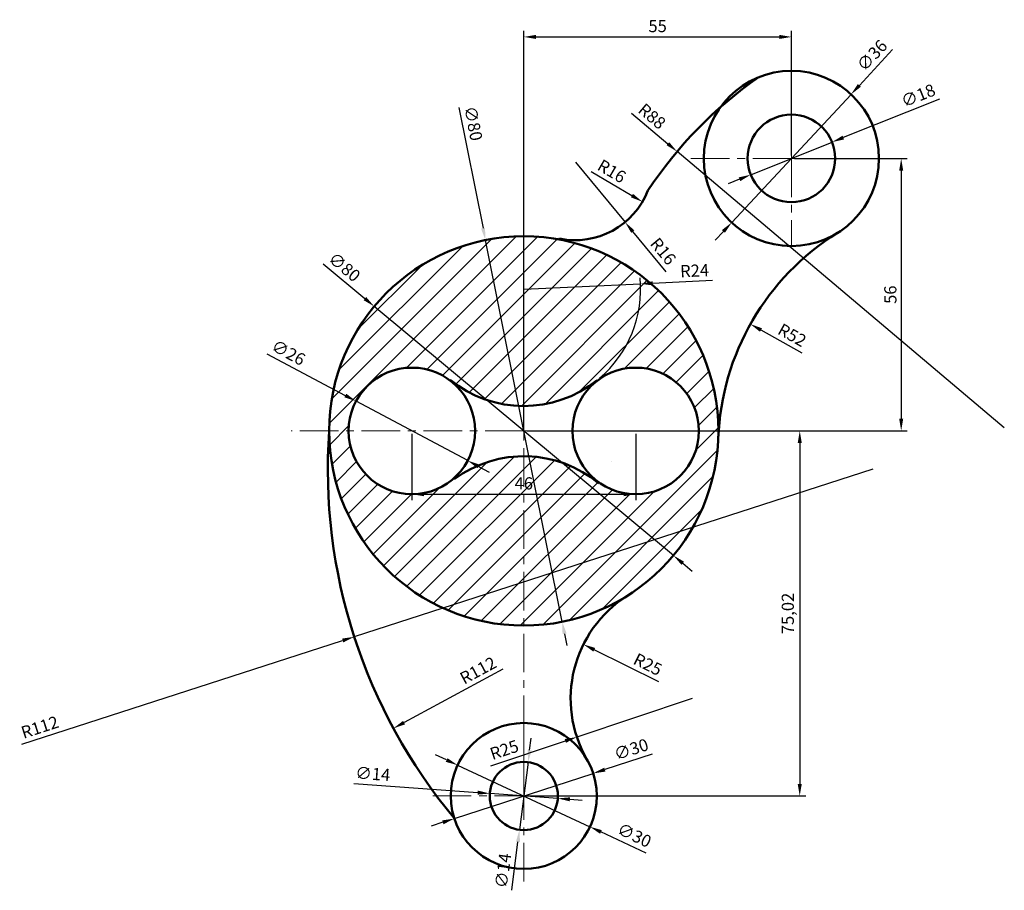
# Model space of a CAD drawing. Units: millimetres. Extents: x 2710 to 2913, y 1178 to 1357.
import ezdxf

# ---------------------------------------------------------------- set-up
doc = ezdxf.new("R2010")
doc.units = ezdxf.units.MM
doc.linetypes.add('CENTER', pattern=[50.8, 31.75, -6.35, 6.35, -6.35])
for name, color, linetype, lineweight in [('M-CNTR', 4, 'CENTER', 18), ('M-DIMS', 2, 'Continuous', 25), ('M-HATC', 8, 'Continuous', 18), ('M-OUTL', 7, 'Continuous', 50)]:
    doc.layers.add(name, color=color, linetype=linetype, lineweight=lineweight)
doc.styles.get("Standard").update_dxf_attribs({"font": 'arial.ttf'})
doc.dimstyles.new('ISO-25', dxfattribs={"dimtxt": 2.5, "dimasz": 2.5, "dimexe": 1.25, "dimexo": 0.625, "dimtad": 1, "dimtxsty": 'Standard', "dimcen": 2.5, "dimadec": 0, "dimazin": 0, "dimtfac": 1, "dimtmove": 0, "dimatfit": 3, "dimfxl": 1, "dimarcsym": 0})

# ---------------------------------------------------------------- blocks, each defined once
blk = doc.blocks.new('*D1')
at = {"layer": 'Defpoints', "color": 0, "transparency": 16777216}
for p in [(2813.89, 1272.64), (2813.89, 1197.62), (2870.6, 1197.62)]:
    blk.add_point(p, dxfattribs=at)
at = {"layer": 'M-DIMS', "color": 0, "lineweight": -2, "transparency": 16777216}
for p, q in [((2814.51, 1272.64), (2871.85, 1272.64)), ((2870.6, 1270.14), (2870.6, 1200.12)), ((2814.51, 1197.62), (2871.85, 1197.62))]:
    blk.add_line(p, q, dxfattribs=at)
at = {"layer": 'M-DIMS', "color": 0, "transparency": 16777216}
for points in [[(2870.18, 1270.14), (2871.02, 1270.14), (2870.6, 1272.64)], [(2870.18, 1200.12), (2871.02, 1200.12), (2870.6, 1197.62)]]:
    blk.add_solid(points, dxfattribs=at)
at = {"layer": 'M-DIMS', "color": 0, "transparency": 16777216, "insert": (2868.47, 1235.13), "char_height": 2.5, "attachment_point": 5, "rotation": 90}
blk.add_mtext('75,02', dxfattribs=at)
blk = doc.blocks.new('*D2')
at = {"layer": 'Defpoints', "color": 0, "transparency": 16777216}
for p in [(2868.89, 1353.61), (2868.89, 1328.64), (2813.89, 1272.64)]:
    blk.add_point(p, dxfattribs=at)
at = {"layer": 'M-DIMS', "color": 0, "lineweight": -2, "transparency": 16777216}
for p, q in [((2813.89, 1273.27), (2813.89, 1354.86)), ((2868.89, 1329.27), (2868.89, 1354.86)), ((2816.39, 1353.61), (2866.39, 1353.61))]:
    blk.add_line(p, q, dxfattribs=at)
at = {"layer": 'M-DIMS', "color": 0, "transparency": 16777216}
for points in [[(2816.39, 1354.03), (2816.39, 1353.19), (2813.89, 1353.61)], [(2866.39, 1354.03), (2866.39, 1353.19), (2868.89, 1353.61)]]:
    blk.add_solid(points, dxfattribs=at)
at = {"layer": 'M-DIMS', "color": 0, "transparency": 16777216, "insert": (2841.39, 1355.51), "char_height": 2.5, "attachment_point": 5}
blk.add_mtext('55', dxfattribs=at)
blk = doc.blocks.new('*D3')
at = {"layer": 'Defpoints', "color": 0, "transparency": 16777216}
for p in [(2868.89, 1328.64), (2813.89, 1272.64), (2891.45, 1272.64)]:
    blk.add_point(p, dxfattribs=at)
at = {"layer": 'M-DIMS', "color": 0, "lineweight": -2, "transparency": 16777216}
for p, q in [((2869.51, 1328.64), (2892.7, 1328.64)), ((2891.45, 1326.14), (2891.45, 1275.14)), ((2814.51, 1272.64), (2892.7, 1272.64))]:
    blk.add_line(p, q, dxfattribs=at)
at = {"layer": 'M-DIMS', "color": 0, "transparency": 16777216}
for points in [[(2891.04, 1326.14), (2891.87, 1326.14), (2891.45, 1328.64)], [(2891.04, 1275.14), (2891.87, 1275.14), (2891.45, 1272.64)]]:
    blk.add_solid(points, dxfattribs=at)
at = {"layer": 'M-DIMS', "color": 0, "transparency": 16777216, "insert": (2889.55, 1300.64), "char_height": 2.5, "attachment_point": 5, "rotation": 90}
blk.add_mtext('56', dxfattribs=at)
blk = doc.blocks.new('*D4')
at = {"layer": 'Defpoints', "color": 0, "transparency": 16777216}
for p in [(2813.89, 1301.75), (2837.86, 1302.86)]:
    blk.add_point(p, dxfattribs=at)
at = {"layer": 'M-DIMS', "color": 0, "lineweight": -2, "transparency": 16777216}
for p, q in [((2852.69, 1303.54), (2840.36, 1302.97)), ((2813.89, 1301.75), (2837.86, 1302.86))]:
    blk.add_line(p, q, dxfattribs=at)
blk.add_arc((2813.89, 1301.75), 24, 310.331, 5.6178, dxfattribs=at)
at = {"layer": 'M-DIMS', "color": 0, "transparency": 16777216}
blk.add_solid([(2840.34, 1303.39), (2840.38, 1302.56), (2837.86, 1302.86)], dxfattribs=at)
at = {"layer": 'M-DIMS', "color": 0, "transparency": 16777216, "insert": (2849, 1305.25), "char_height": 2.5, "attachment_point": 5, "rotation": 2.6336}
blk.add_mtext('R24', dxfattribs=at)
blk = doc.blocks.new('*D5')
at = {"layer": 'Defpoints', "color": 0, "transparency": 16777216}
for p in [(2826.14, 1228.78), (2848.52, 1217.64)]:
    blk.add_point(p, dxfattribs=at)
at = {"layer": 'M-DIMS', "color": 0, "lineweight": -2, "transparency": 16777216}
blk.add_line((2841.64, 1221.06), (2828.38, 1227.67), dxfattribs=at)
at = {"layer": 'M-DIMS', "color": 0, "transparency": 16777216}
blk.add_solid([(2828.57, 1228.04), (2828.19, 1227.29), (2826.14, 1228.78)], dxfattribs=at)
at = {"layer": 'M-DIMS', "color": 0, "transparency": 16777216, "insert": (2839.24, 1224.38), "char_height": 2.5, "attachment_point": 5, "rotation": 333.5253}
blk.add_mtext('R25', dxfattribs=at)
blk = doc.blocks.new('*D6')
at = {"layer": 'Defpoints', "color": 0, "transparency": 16777216}
for p in [(2885.61, 1264.77), (2787.08, 1211.52)]:
    blk.add_point(p, dxfattribs=at)
at = {"layer": 'M-DIMS', "color": 0, "lineweight": -2, "transparency": 16777216}
blk.add_line((2809.55, 1223.66), (2789.28, 1212.71), dxfattribs=at)
at = {"layer": 'M-DIMS', "color": 0, "transparency": 16777216}
blk.add_solid([(2789.08, 1213.07), (2789.47, 1212.34), (2787.08, 1211.52)], dxfattribs=at)
at = {"layer": 'M-DIMS', "color": 0, "transparency": 16777216, "insert": (2804.64, 1223.15), "char_height": 2.5, "attachment_point": 5, "rotation": 28.3886}
blk.add_mtext('R112', dxfattribs=at)
blk = doc.blocks.new('*D7')
at = {"layer": 'Defpoints', "color": 0, "transparency": 16777216}
for p in [(2824.48, 1327.84), (2838.27, 1319.73)]:
    blk.add_point(p, dxfattribs=at)
at = {"layer": 'M-DIMS', "color": 0, "lineweight": -2, "transparency": 16777216}
blk.add_line((2827.74, 1325.93), (2836.12, 1321), dxfattribs=at)
at = {"layer": 'M-DIMS', "color": 0, "transparency": 16777216}
blk.add_solid([(2836.33, 1321.36), (2835.91, 1320.64), (2838.27, 1319.73)], dxfattribs=at)
at = {"layer": 'M-DIMS', "color": 0, "transparency": 16777216, "insert": (2831.81, 1325.74), "char_height": 2.5, "attachment_point": 5, "rotation": 329.5523}
blk.add_mtext('R16', dxfattribs=at)
blk = doc.blocks.new('*D8')
at = {"layer": 'Defpoints', "color": 0, "transparency": 16777216}
for p in [(2845.4, 1330.05), (2912.65, 1273.29)]:
    blk.add_point(p, dxfattribs=at)
at = {"layer": 'M-DIMS', "color": 0, "lineweight": -2, "transparency": 16777216}
for p, q in [((2836.05, 1337.94), (2843.49, 1331.66)), ((2912.65, 1273.29), (2845.4, 1330.05))]:
    blk.add_line(p, q, dxfattribs=at)
at = {"layer": 'M-DIMS', "color": 0, "transparency": 16777216}
blk.add_solid([(2843.76, 1331.98), (2843.22, 1331.35), (2845.4, 1330.05)], dxfattribs=at)
at = {"layer": 'M-DIMS', "color": 0, "transparency": 16777216, "insert": (2840.04, 1337.06), "char_height": 2.5, "attachment_point": 5, "rotation": 319.8348}
blk.add_mtext('R88', dxfattribs=at)
blk = doc.blocks.new('*D9')
at = {"layer": 'Defpoints', "color": 0, "transparency": 16777216}
for p in [(2860.46, 1294.59), (2905.82, 1269.18)]:
    blk.add_point(p, dxfattribs=at)
at = {"layer": 'M-DIMS', "color": 0, "lineweight": -2, "transparency": 16777216}
blk.add_line((2871.1, 1288.63), (2862.64, 1293.37), dxfattribs=at)
at = {"layer": 'M-DIMS', "color": 0, "transparency": 16777216}
blk.add_solid([(2862.84, 1293.74), (2862.43, 1293.01), (2860.46, 1294.59)], dxfattribs=at)
at = {"layer": 'M-DIMS', "color": 0, "transparency": 16777216, "insert": (2868.89, 1292.05), "char_height": 2.5, "attachment_point": 5, "rotation": 330.7397}
blk.add_mtext('R52', dxfattribs=at)
blk = doc.blocks.new('*D10')
at = {"layer": 'Defpoints', "color": 0, "transparency": 16777216}
for p in [(2828.15, 1202.27), (2799.62, 1192.98)]:
    blk.add_point(p, dxfattribs=at)
at = {"layer": 'M-DIMS', "color": 0, "lineweight": -2, "transparency": 16777216}
for p, q in [((2840.25, 1206.21), (2830.53, 1203.04)), ((2799.62, 1192.98), (2828.15, 1202.27)), ((2797.24, 1192.21), (2794.87, 1191.44))]:
    blk.add_line(p, q, dxfattribs=at)
at = {"layer": 'M-DIMS', "color": 0, "transparency": 16777216}
for points in [[(2830.4, 1203.44), (2830.66, 1202.64), (2828.15, 1202.27)], [(2797.12, 1192.61), (2797.37, 1191.81), (2799.62, 1192.98)]]:
    blk.add_solid(points, dxfattribs=at)
at = {"layer": 'M-DIMS', "color": 0, "transparency": 16777216, "insert": (2836.05, 1206.91), "char_height": 2.5, "attachment_point": 5, "rotation": 18.0277}
blk.add_mtext('∅30', dxfattribs=at)
blk = doc.blocks.new('*D11')
at = {"layer": 'Defpoints', "color": 0, "transparency": 16777216}
for p in [(2806.9, 1198.13), (2820.87, 1197.12)]:
    blk.add_point(p, dxfattribs=at)
at = {"layer": 'M-DIMS', "color": 0, "lineweight": -2, "transparency": 16777216}
for p, q in [((2778.93, 1200.16), (2804.41, 1198.31)), ((2820.87, 1197.12), (2806.9, 1198.13)), ((2823.36, 1196.94), (2825.85, 1196.76))]:
    blk.add_line(p, q, dxfattribs=at)
at = {"layer": 'M-DIMS', "color": 0, "transparency": 16777216}
for points in [[(2804.44, 1198.73), (2804.38, 1197.9), (2806.9, 1198.13)], [(2823.39, 1197.35), (2823.33, 1196.52), (2820.87, 1197.12)]]:
    blk.add_solid(points, dxfattribs=at)
at = {"layer": 'M-DIMS', "color": 0, "transparency": 16777216, "insert": (2782.83, 1201.85), "char_height": 2.5, "attachment_point": 5, "rotation": 355.8573}
blk.add_mtext('∅14', dxfattribs=at)
blk = doc.blocks.new('*D12')
at = {"layer": 'Defpoints', "color": 0, "transparency": 16777216}
for p in [(2779.41, 1278.75), (2802.36, 1266.53)]:
    blk.add_point(p, dxfattribs=at)
at = {"layer": 'M-DIMS', "color": 0, "lineweight": -2, "transparency": 16777216}
for p, q in [((2761.1, 1288.49), (2777.2, 1279.92)), ((2802.36, 1266.53), (2779.41, 1278.75)), ((2804.57, 1265.36), (2806.78, 1264.19))]:
    blk.add_line(p, q, dxfattribs=at)
at = {"layer": 'M-DIMS', "color": 0, "transparency": 16777216}
for points in [[(2777.4, 1280.29), (2777.01, 1279.55), (2779.41, 1278.75)], [(2804.77, 1265.73), (2804.37, 1264.99), (2802.36, 1266.53)]]:
    blk.add_solid(points, dxfattribs=at)
at = {"layer": 'M-DIMS', "color": 0, "transparency": 16777216, "insert": (2765.36, 1288.45), "char_height": 2.5, "attachment_point": 5, "rotation": 331.9853}
blk.add_mtext('∅26', dxfattribs=at)
blk = doc.blocks.new('*D13')
at = {"layer": 'Defpoints', "color": 0, "transparency": 16777216}
for p in [(2783.14, 1298.23), (2844.63, 1247.05)]:
    blk.add_point(p, dxfattribs=at)
at = {"layer": 'M-DIMS', "color": 0, "lineweight": -2, "transparency": 16777216}
for p, q in [((2772.65, 1306.97), (2781.22, 1299.83)), ((2844.63, 1247.05), (2783.14, 1298.23)), ((2846.55, 1245.45), (2848.47, 1243.85))]:
    blk.add_line(p, q, dxfattribs=at)
at = {"layer": 'M-DIMS', "color": 0, "transparency": 16777216}
for points in [[(2781.49, 1300.15), (2780.96, 1299.51), (2783.14, 1298.23)], [(2846.82, 1245.77), (2846.28, 1245.13), (2844.63, 1247.05)]]:
    blk.add_solid(points, dxfattribs=at)
at = {"layer": 'M-DIMS', "color": 0, "transparency": 16777216, "insert": (2776.81, 1306.07), "char_height": 2.5, "attachment_point": 5, "rotation": 320.2245}
blk.add_mtext('∅80', dxfattribs=at)
blk = doc.blocks.new('*D14')
at = {"layer": 'Defpoints', "color": 0, "transparency": 16777216}
for p in [(2881.15, 1341.81), (2856.62, 1315.47)]:
    blk.add_point(p, dxfattribs=at)
at = {"layer": 'M-DIMS', "color": 0, "lineweight": -2, "transparency": 16777216}
for p, q in [((2889.7, 1351), (2882.85, 1343.64)), ((2856.62, 1315.47), (2881.15, 1341.81)), ((2854.92, 1313.64), (2853.21, 1311.81))]:
    blk.add_line(p, q, dxfattribs=at)
at = {"layer": 'M-DIMS', "color": 0, "transparency": 16777216}
for points in [[(2882.55, 1343.93), (2883.16, 1343.36), (2881.15, 1341.81)], [(2854.61, 1313.92), (2855.22, 1313.35), (2856.62, 1315.47)]]:
    blk.add_solid(points, dxfattribs=at)
at = {"layer": 'M-DIMS', "color": 0, "transparency": 16777216, "insert": (2885.69, 1349.58), "char_height": 2.5, "attachment_point": 5, "rotation": 47.0445}
blk.add_mtext('∅36', dxfattribs=at)
blk = doc.blocks.new('*D15')
at = {"layer": 'Defpoints', "color": 0, "transparency": 16777216}
for p in [(2877.24, 1331.99), (2860.53, 1325.29)]:
    blk.add_point(p, dxfattribs=at)
at = {"layer": 'M-DIMS', "color": 0, "lineweight": -2, "transparency": 16777216}
for p, q in [((2899.3, 1340.85), (2879.56, 1332.92)), ((2860.53, 1325.29), (2877.24, 1331.99)), ((2858.21, 1324.36), (2855.89, 1323.43))]:
    blk.add_line(p, q, dxfattribs=at)
at = {"layer": 'M-DIMS', "color": 0, "transparency": 16777216}
for points in [[(2879.4, 1333.31), (2879.71, 1332.54), (2877.24, 1331.99)], [(2858.06, 1324.74), (2858.37, 1323.97), (2860.53, 1325.29)]]:
    blk.add_solid(points, dxfattribs=at)
at = {"layer": 'M-DIMS', "color": 0, "transparency": 16777216, "insert": (2895.06, 1341.27), "char_height": 2.5, "attachment_point": 5, "rotation": 21.8728}
blk.add_mtext('∅18', dxfattribs=at)
blk = doc.blocks.new('*D16')
at = {"layer": 'Defpoints', "color": 0, "transparency": 16777216}
for p in [(2790.89, 1272.64), (2836.89, 1272.64), (2836.89, 1259.64)]:
    blk.add_point(p, dxfattribs=at)
at = {"layer": 'M-DIMS', "color": 0, "lineweight": -2, "transparency": 16777216}
for p, q in [((2790.89, 1272.02), (2790.89, 1258.39)), ((2836.89, 1272.02), (2836.89, 1258.39)), ((2793.39, 1259.64), (2834.39, 1259.64))]:
    blk.add_line(p, q, dxfattribs=at)
at = {"layer": 'M-DIMS', "color": 0, "transparency": 16777216}
for points in [[(2793.39, 1260.06), (2793.39, 1259.22), (2790.89, 1259.64)], [(2834.39, 1260.06), (2834.39, 1259.22), (2836.89, 1259.64)]]:
    blk.add_solid(points, dxfattribs=at)
at = {"layer": 'M-DIMS', "color": 0, "transparency": 16777216, "insert": (2813.89, 1261.54), "char_height": 2.5, "attachment_point": 5}
blk.add_mtext('46', dxfattribs=at)
blk = doc.blocks.new('*D17')
at = {"layer": 'Defpoints', "color": 0, "transparency": 16777216}
for p in [(2806, 1311.86), (2821.77, 1233.43)]:
    blk.add_point(p, dxfattribs=at)
at = {"layer": 'M-DIMS', "color": 0, "lineweight": -2, "transparency": 16777216}
for p, q in [((2800.53, 1339.08), (2805.51, 1314.31)), ((2821.77, 1233.43), (2806, 1311.86)), ((2822.26, 1230.97), (2822.76, 1228.52))]:
    blk.add_line(p, q, dxfattribs=at)
at = {"layer": 'M-DIMS', "color": 0, "transparency": 16777216}
for points in [[(2805.92, 1314.39), (2805.1, 1314.22), (2806, 1311.86)], [(2822.67, 1231.06), (2821.85, 1230.89), (2821.77, 1233.43)]]:
    blk.add_solid(points, dxfattribs=at)
at = {"layer": 'M-DIMS', "color": 0, "transparency": 16777216, "insert": (2803.2, 1335.77), "char_height": 2.5, "attachment_point": 5, "rotation": 281.3684}
blk.add_mtext('∅80', dxfattribs=at)
blk = doc.blocks.new('*D18')
at = {"layer": 'Defpoints', "color": 0, "transparency": 16777216}
for p in [(2800.29, 1203.96), (2827.48, 1191.29)]:
    blk.add_point(p, dxfattribs=at)
at = {"layer": 'M-DIMS', "color": 0, "lineweight": -2, "transparency": 16777216}
for p, q in [((2798.02, 1205.02), (2795.76, 1206.07)), ((2800.29, 1203.96), (2827.48, 1191.29)), ((2839.06, 1185.89), (2829.75, 1190.23))]:
    blk.add_line(p, q, dxfattribs=at)
at = {"layer": 'M-DIMS', "color": 0, "transparency": 16777216}
for points in [[(2798.2, 1205.39), (2797.85, 1204.64), (2800.29, 1203.96)], [(2829.92, 1190.61), (2829.57, 1189.86), (2827.48, 1191.29)]]:
    blk.add_solid(points, dxfattribs=at)
at = {"layer": 'M-DIMS', "color": 0, "transparency": 16777216, "insert": (2836.47, 1189.27), "char_height": 2.5, "attachment_point": 5, "rotation": 335.0157}
blk.add_mtext('∅30', dxfattribs=at)
blk = doc.blocks.new('*D19')
at = {"layer": 'Defpoints', "color": 0, "transparency": 16777216}
for p in [(2814.77, 1204.57), (2813, 1190.68)]:
    blk.add_point(p, dxfattribs=at)
at = {"layer": 'M-DIMS', "color": 0, "lineweight": -2, "transparency": 16777216}
for p, q in [((2815.09, 1207.05), (2815.4, 1209.53)), ((2814.77, 1204.57), (2813, 1190.68)), ((2811.41, 1178.24), (2812.68, 1188.2))]:
    blk.add_line(p, q, dxfattribs=at)
at = {"layer": 'M-DIMS', "color": 0, "transparency": 16777216}
for points in [[(2814.67, 1207.1), (2815.5, 1207), (2814.77, 1204.57)], [(2812.27, 1188.25), (2813.1, 1188.15), (2813, 1190.68)]]:
    blk.add_solid(points, dxfattribs=at)
at = {"layer": 'M-DIMS', "color": 0, "transparency": 16777216, "insert": (2809.94, 1182.23), "char_height": 2.5, "attachment_point": 5, "rotation": 82.7337}
blk.add_mtext('∅14', dxfattribs=at)
blk = doc.blocks.new('*D20')
at = {"layer": 'Defpoints', "color": 0, "transparency": 16777216}
for p in [(2885.61, 1264.77), (2779.03, 1230.33)]:
    blk.add_point(p, dxfattribs=at)
at = {"layer": 'M-DIMS', "color": 0, "lineweight": -2, "transparency": 16777216}
for p, q in [((2885.61, 1264.77), (2779.03, 1230.33)), ((2710.74, 1208.27), (2776.65, 1229.57))]:
    blk.add_line(p, q, dxfattribs=at)
at = {"layer": 'M-DIMS', "color": 0, "transparency": 16777216}
blk.add_solid([(2776.53, 1229.96), (2776.78, 1229.17), (2779.03, 1230.33)], dxfattribs=at)
at = {"layer": 'M-DIMS', "color": 0, "transparency": 16777216, "insert": (2714.51, 1211.46), "char_height": 2.5, "attachment_point": 5, "rotation": 17.9049}
blk.add_mtext('R112', dxfattribs=at)
blk = doc.blocks.new('*D21')
at = {"layer": 'Defpoints', "color": 0, "transparency": 16777216}
for p in [(2848.52, 1217.64), (2824.8, 1209.73)]:
    blk.add_point(p, dxfattribs=at)
at = {"layer": 'M-DIMS', "color": 0, "lineweight": -2, "transparency": 16777216}
for p, q in [((2848.52, 1217.64), (2824.8, 1209.73)), ((2807.14, 1203.85), (2822.43, 1208.94))]:
    blk.add_line(p, q, dxfattribs=at)
at = {"layer": 'M-DIMS', "color": 0, "transparency": 16777216}
blk.add_solid([(2822.3, 1209.34), (2822.56, 1208.55), (2824.8, 1209.73)], dxfattribs=at)
at = {"layer": 'M-DIMS', "color": 0, "transparency": 16777216, "insert": (2809.97, 1206.8), "char_height": 2.5, "attachment_point": 5, "rotation": 18.4273}
blk.add_mtext('R25', dxfattribs=at)
blk = doc.blocks.new('*D22')
at = {"layer": 'Defpoints', "color": 0, "transparency": 16777216}
for p in [(2824.48, 1327.84), (2834.7, 1315.53)]:
    blk.add_point(p, dxfattribs=at)
at = {"layer": 'M-DIMS', "color": 0, "lineweight": -2, "transparency": 16777216}
for p, q in [((2824.48, 1327.84), (2834.7, 1315.53)), ((2843.13, 1305.36), (2836.29, 1313.6))]:
    blk.add_line(p, q, dxfattribs=at)
at = {"layer": 'M-DIMS', "color": 0, "transparency": 16777216}
blk.add_solid([(2836.61, 1313.87), (2835.97, 1313.34), (2834.7, 1315.53)], dxfattribs=at)
at = {"layer": 'M-DIMS', "color": 0, "transparency": 16777216, "insert": (2842.29, 1309.35), "char_height": 2.5, "attachment_point": 5, "rotation": 309.6734}
blk.add_mtext('R16', dxfattribs=at)

msp = doc.modelspace()

# ---------------------------------------------------------------- hatches: boundary and pattern name
at = {"layer": 'M-HATC'}
h = msp.add_hatch(dxfattribs=at)
h.set_pattern_fill('ANSI31', color=256)
h.paths.add_polyline_path([(2813.885, 1312.641, 0.4142136), (2773.885, 1272.641), (2777.885, 1272.641, -0.6180168), (2798.685, 1283.041), (2798.74, 1283.137, 0.1724052), (2813.885, 1277.755)])
h.paths.add_polyline_path([(2813.885, 1312.641), (2813.885, 1277.755, 0.1711078), (2828.937, 1283.061), (2829.01, 1282.984, -0.6205581), (2849.885, 1272.641), (2853.885, 1272.641, 0.4142136)])
h.paths.add_polyline_path([(2813.885, 1267.437, 0.1606543), (2799.607, 1262.728), (2799.503, 1262.908, -0.6464539), (2777.885, 1272.641), (2773.885, 1272.641, 0.4142136), (2813.885, 1232.641)])
h.paths.add_polyline_path([(2853.885, 1272.641), (2849.885, 1272.641, -0.6084748), (2829.377, 1262.028), (2829.276, 1261.853, 0.1758199), (2813.885, 1267.437), (2813.885, 1232.641, 0.4142136)])

# ---------------------------------------------------------------- linework, layer by layer
at = {"layer": 'M-CNTR', "ltscale": 0.25}
for p, q in [((2868.885, 1328.641), (2868.885, 1349.816)), ((2868.885, 1328.641), (2846.755, 1328.641)), ((2868.885, 1328.641), (2891.639, 1328.641)), ((2868.885, 1328.641), (2868.885, 1310.641)), ((2813.885, 1272.641), (2813.885, 1316.947)), ((2813.885, 1272.641), (2766.058, 1272.641)), ((2813.885, 1197.641), (2813.885, 1272.641)), ((2813.885, 1272.641), (2868.885, 1272.641)), ((2813.885, 1180.025), (2813.885, 1215.256)), ((2795.154, 1197.625), (2831.952, 1197.625))]:
    msp.add_line(p, q, dxfattribs=at)
at = {"layer": 'M-CNTR'}
msp.add_line((2813.885, 1272.641), (2860.975, 1272.641), dxfattribs=at)
at = {"layer": 'M-OUTL'}
for p, q in [((2821.221, 1312.177), (2820.989, 1312.005)), ((2798.685, 1283.041), (2798.74, 1283.137)), ((2829.01, 1282.984), (2828.937, 1283.061)), ((2831.827, 1266.27), (2831.827, 1266.27)), ((2799.607, 1262.728), (2799.503, 1262.908)), ((2829.276, 1261.853), (2829.377, 1262.028))]:
    msp.add_line(p, q, dxfattribs=at)
for centre, radius in [((2868.885, 1328.641), 18), ((2868.885, 1328.641), 9), ((2813.885, 1272.641), 40), ((2790.885, 1272.641), 13), ((2836.885, 1272.641), 13), ((2813.885, 1197.625), 15), ((2813.885, 1197.625), 7)]:
    msp.add_circle(centre, radius, dxfattribs=at)
for centre, radius, start, end in [((2912.647, 1273.292), 88, 125.0954, 146.33428), ((2824.481, 1327.841), 16, 258.24363, 338.87385), ((2905.82, 1269.178), 52, 121.84615, 177.84295), ((2813.885, 1301.755), 24, 230.87229, 308.83888), ((2885.608, 1264.767), 112, 175.96873, 219.84101), ((2813.885, 1243.437), 24, 50.11271, 126.50731), ((2848.52, 1217.636), 25, 122.19717, 210.0194)]:
    msp.add_arc(centre, radius, start, end, dxfattribs=at)

# ---------------------------------------------------------------- dimensions: what is measured, and where the dimension line sits
at = {"layer": 'M-DIMS'}
for base, p1, p2, picture, middle in [((2868.885, 1353.611), (2813.885, 1272.641), (2868.885, 1328.641), '*D2', (2841.385, 1355.507)), ((2836.885, 1259.641), (2790.885, 1272.641), (2836.885, 1272.641), '*D16', (2813.885, 1261.542))]:
    dim = msp.add_linear_dim(base=base, p1=p1, p2=p2, dimstyle='ISO-25', override={"dimclrd": 0, "dimclre": 0, "dimclrt": 0}, dxfattribs=at)
    dim.commit()
    dim.dimension.update_dxf_attribs({"geometry": picture, "text_midpoint": middle})
dim = msp.add_diameter_dim_2p(p1=(2856.62, 1315.467), p2=(2881.151, 1341.815), dimstyle='ISO-25', override={"dimclrd": 0, "dimclre": 0, "dimclrt": 0}, dxfattribs=at)
dim.commit()
dim.dimension.update_dxf_attribs({"geometry": '*D14', "text_midpoint": (2885.688, 1349.58)})
for p1, p2, override, picture, middle in [((2860.533, 1325.288), (2877.238, 1331.994), {"dimclrd": 0, "dimclre": 0, "dimclrt": 0}, '*D15', (2895.796, 1339.444)), ((2821.77, 1233.425), (2806.001, 1311.856), {"dimdec": 0, "dimlfac": 1, "dimrnd": 0, "dimzin": 0, "dimdsep": 46, "dimlunit": 2}, '*D17', (2801.27, 1335.385)), ((2844.628, 1247.049), (2783.143, 1298.232), {"dimclrd": 0, "dimclre": 0, "dimclrt": 0}, '*D13', (2775.549, 1304.554)), ((2802.362, 1266.535), (2779.409, 1278.747), {"dimclrd": 0, "dimclre": 0, "dimclrt": 0}, '*D12', (2764.437, 1286.712)), ((2799.622, 1192.983), (2828.149, 1202.267), {"dimclrd": 0, "dimclre": 0, "dimclrt": 0}, '*D10', (2836.664, 1205.038)), ((2814.771, 1204.568), (2813, 1190.681), {"dimdec": 0, "dimlfac": 1, "dimrnd": 0, "dimzin": 0, "dimdsep": 46, "dimlunit": 2}, '*D19', (2811.891, 1181.981)), ((2800.289, 1203.96), (2827.482, 1191.289), {"dimdec": 0, "dimlfac": 1, "dimrnd": 0, "dimzin": 0, "dimdsep": 46, "dimlunit": 2}, '*D18', (2835.64, 1187.488)), ((2820.867, 1197.119), (2806.904, 1198.13), {"dimclrd": 0, "dimclre": 0, "dimclrt": 0}, '*D11', (2782.692, 1199.884))]:
    dim = msp.add_diameter_dim_2p(p1=p1, p2=p2, dimstyle='ISO-25', override=override, dxfattribs=at)
    dim.commit()
    dim.dimension.update_dxf_attribs({"geometry": picture, "text_midpoint": middle, "dimtype": 163})
dim = msp.add_radius_dim(center=(2912.647, 1273.292), mpoint=(2845.398, 1330.051), dimstyle='ISO-25', override={"dimclrd": 0, "dimclre": 0, "dimclrt": 0}, dxfattribs=at)
dim.commit()
dim.dimension.update_dxf_attribs({"geometry": '*D8', "text_midpoint": (2840.041, 1337.061)})
for base, p1, p2, picture, middle in [((2891.454, 1272.641), (2868.885, 1328.641), (2813.885, 1272.641), '*D3', (2889.552, 1300.641)), ((2870.6, 1197.625), (2813.885, 1272.641), (2813.885, 1197.625), '*D1', (2868.472, 1235.133))]:
    dim = msp.add_linear_dim(base=base, p1=p1, p2=p2, angle=90, dimstyle='ISO-25', override={"dimclrd": 0, "dimclre": 0, "dimclrt": 0}, dxfattribs=at)
    dim.commit()
    dim.dimension.update_dxf_attribs({"geometry": picture, "text_midpoint": middle})
for center, mpoint, override, picture, middle in [((2824.481, 1327.841), (2838.274, 1319.733), {"dimclrd": 0, "dimclre": 0, "dimclrt": 0}, '*D7', (2830.851, 1324.097)), ((2824.481, 1327.841), (2834.695, 1315.526), {"dimdec": 0, "dimlfac": 1, "dimrnd": 0, "dimzin": 0, "dimdsep": 46, "dimlunit": 2}, '*D22', (2840.824, 1308.137)), ((2813.885, 1301.755), (2837.86, 1302.857), {"dimclrd": 0, "dimclre": 0, "dimclrt": 0}, '*D4', (2849.087, 1303.374)), ((2905.82, 1269.178), (2860.455, 1294.594), {"dimclrd": 0, "dimclre": 0, "dimclrt": 0}, '*D9', (2867.957, 1290.391)), ((2885.608, 1264.767), (2779.033, 1230.334), {"dimdec": 0, "dimlfac": 1, "dimrnd": 0, "dimzin": 0, "dimdsep": 46, "dimlunit": 2}, '*D20', (2715.087, 1209.674)), ((2885.608, 1264.767), (2787.077, 1211.517), {"dimclrd": 0, "dimclre": 0, "dimclrt": 0}, '*D6', (2805.533, 1221.491)), ((2848.52, 1217.636), (2826.141, 1228.781), {"dimclrd": 0, "dimclre": 0, "dimclrt": 0}, '*D5', (2838.397, 1222.678)), ((2848.52, 1217.636), (2824.802, 1209.734), {"dimdec": 0, "dimlfac": 1, "dimrnd": 0, "dimzin": 0, "dimdsep": 46, "dimlunit": 2}, '*D21', (2810.571, 1204.992))]:
    dim = msp.add_radius_dim(center=center, mpoint=mpoint, dimstyle='ISO-25', override=override, dxfattribs=at)
    dim.commit()
    dim.dimension.update_dxf_attribs({"geometry": picture, "text_midpoint": middle, "dimtype": 164})

doc.saveas('drawing.dxf')
